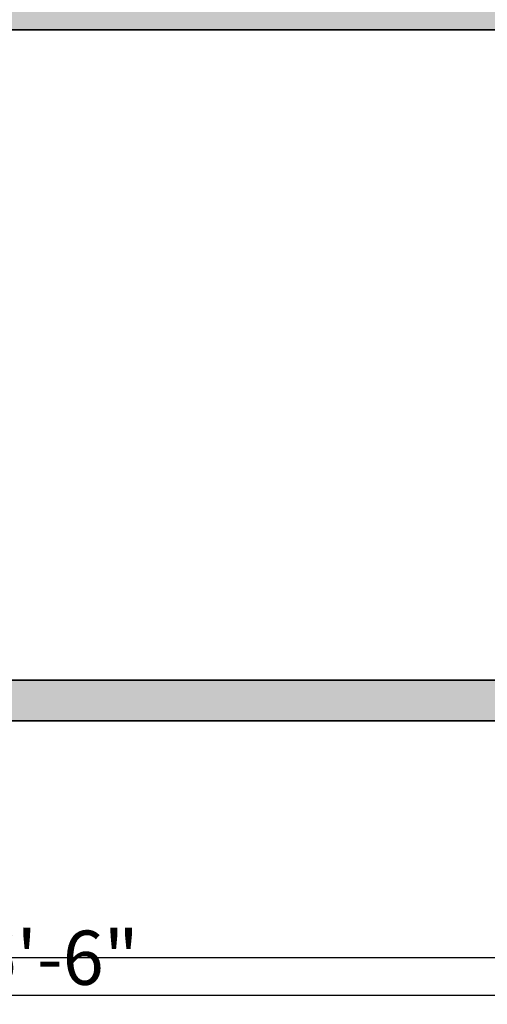
# Model space of a CAD drawing. Units: inches. Extents: x 2083 to 3317, y 1141 to 2115.
# Tile 84 of 256: x 2382 to 2486, y 1201 to 1419. Entities that reach past the tile are written whole.
import ezdxf

# ---------------------------------------------------------------- set-up
doc = ezdxf.new("R2010")
doc.units = ezdxf.units.IN
doc.layers.add('A-ANNO-DIMS', color=2, linetype='Continuous', lineweight=18)
doc.layers.add('A-WALL', color=7, linetype='Continuous', lineweight=35)
doc.layers.add('A-WALL-PATT', color=251, linetype='Continuous', lineweight=13, true_color=0x636466)
doc.styles.get("Standard").update_dxf_attribs({"font": 'arial.ttf'})
doc.dimstyles.new('ISO-25', dxfattribs={"dimtxt": 12, "dimasz": 12, "dimexe": 1.25, "dimexo": 0.625, "dimtad": 1, "dimlunit": 3, "dimtxsty": 'Standard', "dimcen": 2.5, "dimadec": 0, "dimazin": 0, "dimtfac": 1, "dimtmove": 0, "dimatfit": 3, "dimfxl": 1, "dimarcsym": 0})

# ---------------------------------------------------------------- blocks, each defined once
blk = doc.blocks.new('*D12')
at = {"layer": 'A-ANNO-DIMS', "color": 0, "lineweight": -2, "transparency": 16777216}
for p, q in [((2226.96, 1262.64), (2226.96, 1201.28)), ((2544.96, 1262.64), (2544.96, 1201.28)), ((2238.96, 1202.53), (2532.96, 1202.53))]:
    blk.add_line(p, q, dxfattribs=at)
at = {"layer": 'A-ANNO-DIMS', "color": 0, "transparency": 16777216}
for points in [[(2238.96, 1204.53), (2238.96, 1200.53), (2226.96, 1202.53)], [(2532.96, 1204.53), (2532.96, 1200.53), (2544.96, 1202.53)]]:
    blk.add_solid(points, dxfattribs=at)
at = {"layer": 'Defpoints', "color": 0, "transparency": 16777216}
for p in [(2226.96, 1263.26), (2544.96, 1263.26), (2544.96, 1202.53)]:
    blk.add_point(p, dxfattribs=at)
at = {"layer": 'A-ANNO-DIMS', "color": 0, "transparency": 16777216, "insert": (2385.96, 1209.29), "char_height": 12, "attachment_point": 5}
blk.add_mtext('26\'-6"', dxfattribs=at)
blk = doc.blocks.new('*D30')
at = {"layer": 'A-ANNO-DIMS', "color": 0, "lineweight": -2, "transparency": 16777216}
for p, q in [((2240.02, 1445.27), (2240.02, 1448.05)), ((2254.33, 1445.27), (2254.33, 1448.05)), ((2228.02, 1446.8), (2216.02, 1446.8)), ((2240.02, 1446.8), (2254.33, 1446.8)), ((2266.33, 1446.8), (2413.76, 1446.8))]:
    blk.add_line(p, q, dxfattribs=at)
at = {"layer": 'A-ANNO-DIMS', "color": 0, "transparency": 16777216}
for points in [[(2228.02, 1448.8), (2228.02, 1444.8), (2240.02, 1446.8)], [(2266.33, 1448.8), (2266.33, 1444.8), (2254.33, 1446.8)]]:
    blk.add_solid(points, dxfattribs=at)
at = {"layer": 'Defpoints', "color": 0, "transparency": 16777216}
for p in [(2254.33, 1446.8), (2240.02, 1444.65), (2254.33, 1444.65)]:
    blk.add_point(p, dxfattribs=at)
at = {"layer": 'A-ANNO-DIMS', "color": 0, "transparency": 16777216, "insert": (2346.05, 1453.63), "char_height": 12, "attachment_point": 5}
blk.add_mtext('WC 1\'-2 1/2" TYP.', dxfattribs=at)
blk = doc.blocks.new('*D34')
at = {"layer": 'A-ANNO-DIMS', "color": 0, "lineweight": -2, "transparency": 16777216}
for p, q in [((2226.96, 1262.64), (2226.96, 1209.66)), ((3126.96, 1262.64), (3126.96, 1209.66)), ((2238.96, 1210.91), (3114.96, 1210.91))]:
    blk.add_line(p, q, dxfattribs=at)
at = {"layer": 'A-ANNO-DIMS', "color": 0, "transparency": 16777216}
for points in [[(2238.96, 1212.91), (2238.96, 1208.91), (2226.96, 1210.91)], [(3114.96, 1212.91), (3114.96, 1208.91), (3126.96, 1210.91)]]:
    blk.add_solid(points, dxfattribs=at)
at = {"layer": 'Defpoints', "color": 0, "transparency": 16777216}
for p in [(2226.96, 1263.26), (3126.96, 1263.26), (3126.96, 1210.91)]:
    blk.add_point(p, dxfattribs=at)
at = {"layer": 'A-ANNO-DIMS', "color": 0, "transparency": 16777216, "insert": (2676.96, 1217.66), "char_height": 12, "attachment_point": 5}
blk.add_mtext('75\'-0"', dxfattribs=at)

msp = doc.modelspace()

# ---------------------------------------------------------------- hatches: boundary and pattern name
at = {"layer": 'A-WALL-PATT'}
h = msp.add_hatch(color=256, dxfattribs=at)
h.dxf.hatch_style = 1
h.paths.add_polyline_path([(3126.96, 2020.761), (2748.96, 2020.761), (2604.96, 2020.761), (2226.96, 2020.761), (2226.96, 1702.761), (2466.96, 1702.761), (2466.96, 1582.761), (2418.96, 1582.761), (2418.96, 1477.761), (2226.96, 1477.761), (2226.96, 1263.261), (2544.96, 1263.261), (2544.96, 1411.761), (2604.96, 1411.761), (2685.96, 1411.761), (2685.96, 1420.761), (2604.96, 1420.761), (2604.96, 1573.761), (2604.96, 1702.761), (2604.96, 2011.761), (2748.96, 2011.761), (2748.96, 1702.761), (2862.96, 1702.761), (2862.96, 1621.761), (2871.96, 1621.761), (2871.96, 1702.761), (2883.96, 1702.761), (2883.96, 1706.939, -0.0264593), (2883.96, 1711.761), (2757.96, 1711.761), (2757.96, 1807.761), (2787.96, 1807.761), (2787.96, 1812.261), (2757.96, 1812.261), (2757.96, 2011.761), (2877.96, 2011.761), (2877.96, 1812.261), (2847.96, 1812.261), (2847.96, 1807.761), (2889.836, 1807.761), (2889.836, 1812.261), (2882.46, 1812.261), (2882.46, 2011.761), (3117.96, 2011.761), (3117.96, 1812.261), (2937.836, 1812.261), (2937.836, 1807.761), (2995.71, 1807.761), (2995.71, 1796.118), (3000.21, 1796.118), (3000.21, 1807.761), (3117.96, 1807.761), (3117.96, 1711.761), (3000.21, 1711.761), (3000.21, 1760.118), (2998.573, 1760.118, -0.020711), (2995.71, 1760.118), (2995.71, 1711.761), (2931.96, 1711.761), (2931.96, 1702.761), (3126.96, 1702.761)])
h.paths.add_polyline_path([(2471.46, 2011.761), (2471.46, 1810.011), (2462.717, 1810.011), (2462.717, 1805.511), (2505.96, 1805.511), (2505.96, 1810.011), (2475.96, 1810.011), (2475.96, 2011.761), (2595.96, 2011.761), (2595.96, 1810.011), (2565.96, 1810.011), (2565.96, 1805.511), (2595.96, 1805.511), (2595.96, 1711.761), (2235.96, 1711.761), (2235.96, 1805.511), (2353.71, 1805.511), (2353.71, 1796.054), (2358.21, 1796.054), (2358.21, 1805.511), (2414.717, 1805.511), (2414.717, 1810.011), (2235.96, 1810.011), (2235.96, 2011.761)], flags=16)
h.paths.add_polyline_path([(2270.205, 1994.61), (2270.205, 1970.61), (2246.205, 1970.61), (2246.205, 1994.61)], flags=0)
edge = h.paths.add_edge_path(flags=0)
edge.add_ellipse((2332.027, 1899.798), major_axis=(-3.043, 3.043), ratio=0.1682525, start_angle=-161.33217, end_angle=-156.30711, ccw=False)
edge.add_ellipse((2333.082, 1898.744), major_axis=(-1.055, 1.055), ratio=0.4535321, start_angle=-123.37102, end_angle=-94.15911)
edge = h.paths.add_edge_path(flags=0)
edge.add_ellipse((2332.027, 1968.876), major_axis=(3.043, 3.043), ratio=0.1682525, start_angle=18.66783, end_angle=23.69289)
edge.add_spline(control_points=[(2332.926, 1970.691), (2332.227, 1970.336), (2330.894, 1969.659), (2328.413, 1970.932), (2327.204, 1967.749), (2324.71, 1969.956), (2322.533, 1967.012), (2320.013, 1971.296), (2317.68, 1968.158), (2316.041, 1967.102), (2315.427, 1966.81)], knot_values=[0, 0, 0, 0, 2.2670587, 4.3245589, 6.6855835, 8.8786411, 11.121502, 14.300359, 17.7552837, 19.732645, 19.732645, 19.732645, 19.732645], degree=3, periodic=0)
edge.add_ellipse((2332.027, 1968.876), major_axis=(3.043, 3.043), ratio=0.1682525, start_angle=18.66783, end_angle=23.69289, ccw=False)
edge.add_ellipse((2333.082, 1969.931), major_axis=(1.055, 1.055), ratio=0.4535321, start_angle=56.62898, end_angle=85.84089, ccw=False)
edge = h.paths.add_edge_path(flags=0)
edge.add_spline(control_points=[(2296.428, 1967.988), (2293.628, 1965.336), (2287.704, 1959.727), (2299.744, 1949.996), (2294.533, 1935.669), (2290.573, 1920.604), (2293.394, 1909.974), (2296.185, 1904.967)], knot_values=[0.0991853, 0.0991853, 0.0991853, 0.0991853, 0.3453009, 0.6198217, 0.9826526, 1.3860932, 1.8105546, 1.8105546, 1.8105546, 1.8105546], degree=3, periodic=0)
edge.add_spline(control_points=[(2296.185, 1904.967), (2297.384, 1902.619), (2298.001, 1901.949), (2298.553, 1901.468)], knot_values=[0.0062457, 0.0062457, 0.0062457, 0.0062457, 0.0554759, 0.0554759, 0.0554759, 0.0554759], degree=3, periodic=0)
edge.add_spline(control_points=[(2298.553, 1901.468), (2297.259, 1900.923), (2295.225, 1900.232), (2293.06, 1900.614), (2292.101, 1900.788), (2292.09, 1900.791)], knot_values=[0.3128349, 0.3128349, 0.3128349, 0.3128349, 0.4017797, 0.4749867, 0.4759027, 0.4759027, 0.4759027, 0.4759027], degree=3, periodic=0)
edge.add_arc((2292.794, 1904.664), 3.937, 215.4209, 259.69818, ccw=False)
edge.add_spline(control_points=[(2289.585, 1902.382), (2289.477, 1902.535), (2289.368, 1902.688), (2289.261, 1902.841)], knot_values=[0.1028719, 0.1028719, 0.1028719, 0.1028719, 0.1168958, 0.1168958, 0.1168958, 0.1168958], degree=3, periodic=0)
edge.add_spline(control_points=[(2289.261, 1902.841), (2288.687, 1902.55), (2287.64, 1902.02), (2285.881, 1901.874), (2283.853, 1901.504), (2281.72, 1899.711), (2278.467, 1899.493), (2276.157, 1901.883), (2272.259, 1899.804), (2267.778, 1901.843), (2262.244, 1900.184), (2257.415, 1901.782), (2254.318, 1900.726), (2253.178, 1900.337)], knot_values=[0, 0, 0, 0, 1.9079767, 3.4771759, 5.261074, 7.9728515, 11.6802485, 13.7179214, 16.9395917, 22.789562, 27.5025027, 33.5952153, 37.1456181, 37.1456181, 37.1456181, 37.1456181], degree=3, periodic=0)
edge.add_line((2253.178, 1900.337), (2250.244, 1902.841))
edge.add_line((2250.244, 1902.841), (2250.244, 1965.833))
edge.add_line((2250.244, 1965.833), (2253.178, 1968.337))
edge.add_spline(control_points=[(2253.178, 1968.337), (2254.318, 1967.948), (2257.415, 1966.892), (2262.244, 1968.49), (2267.778, 1966.831), (2271.527, 1968.537), (2273.876, 1967.828), (2274.207, 1967.728)], knot_values=[0, 0, 0, 0, 0.0901802, 0.2449351, 0.3646438, 0.5132331, 0.5378548, 0.5378548, 0.5378548, 0.5378548], degree=3, periodic=0)
edge.add_arc((2274.353, 1963.793), 3.937, 72.05113, 92.12795, ccw=False)
edge.add_arc((2281.297, 1985.23), 18.596, 252.05113, 288.56572)
edge.add_arc((2292.317, 1956.029), 12.646, 71.02679, 113.77822, ccw=False)
edge = h.paths.add_edge_path(flags=0)
edge.add_spline(control_points=[(2274.899, 1951.856), (2275.066, 1951.617), (2275.233, 1951.377), (2275.398, 1951.136)], knot_values=[1.4099157, 1.4099157, 1.4099157, 1.4099157, 1.4315903, 1.4315903, 1.4315903, 1.4315903], degree=3, periodic=0)
edge.add_spline(control_points=[(2275.398, 1951.136), (2275.792, 1950.562), (2276.179, 1949.984), (2276.546, 1949.397)], knot_values=[1.3582378, 1.3582378, 1.3582378, 1.3582378, 1.4099157, 1.4099157, 1.4099157, 1.4099157], degree=3, periodic=0)
edge.add_line((2276.546, 1949.397), (2277.437, 1947.862))
edge.add_spline(control_points=[(2277.437, 1947.862), (2276.304, 1945.673), (2274.64, 1942.427), (2274.632, 1938.094), (2272.799, 1930.852), (2274.356, 1943.897), (2275.948, 1947.923), (2276.546, 1949.397)], knot_values=[0.0056315, 0.0056315, 0.0056315, 0.0056315, 0.1860139, 0.2660015, 0.3570872, 0.5963902, 0.7397317, 0.7397317, 0.7397317, 0.7397317], degree=3, periodic=0)
edge.add_spline(control_points=[(2276.546, 1949.397), (2276.179, 1949.984), (2275.792, 1950.562), (2275.398, 1951.136)], knot_values=[1.3582378, 1.3582378, 1.3582378, 1.3582378, 1.4099157, 1.4099157, 1.4099157, 1.4099157], degree=3, periodic=0)
edge.add_spline(control_points=[(2275.398, 1951.136), (2274.943, 1950.08), (2274.208, 1948.025), (2273.935, 1944.851), (2272.469, 1937.627), (2273.466, 1945.696), (2274.701, 1951.059), (2274.899, 1951.856)], knot_values=[0.1043639, 0.1043639, 0.1043639, 0.1043639, 0.1896363, 0.2696239, 0.3607096, 0.6000126, 0.6446217, 0.6446217, 0.6446217, 0.6446217], degree=3, periodic=0)
h.paths.add_polyline_path([(2269.168, 1963.128, -0.3575267), (2268.171, 1960.976, -0.0925607), (2268.171, 1939.436, -0.3575267), (2269.168, 1937.285, -0.3575267), (2267.016, 1938.282, -0.1647847), (2254.686, 1938.282, -0.3575267), (2252.534, 1937.285, -0.3575267), (2253.531, 1939.436, -0.0925607), (2253.531, 1960.976, -0.3575267), (2252.534, 1963.128, -0.3575267), (2254.686, 1962.131, -0.1647847), (2267.016, 1962.131, -0.3575267)], flags=0)
h.paths.add_polyline_path([(2248.874, 1967.802), (2248.874, 1957.028), (2249.458, 1957.028), (2249.458, 1911.647), (2248.874, 1911.647), (2248.874, 1900.873), (2246.512, 1900.873, 0.1973271), (2244.15, 1902.457), (2244.15, 1966.218, 0.1973271), (2246.512, 1967.802)], flags=0)
h.paths.add_polyline_path([(2269.168, 1931.389, -0.3575267), (2268.171, 1929.238, -0.0925607), (2268.171, 1907.698, -0.3575267), (2269.168, 1905.547, -0.3575267), (2267.016, 1906.544, -0.1647847), (2254.686, 1906.544, -0.3575267), (2252.534, 1905.547, -0.3575267), (2253.531, 1907.698, -0.0925607), (2253.531, 1929.238, -0.3575267), (2252.534, 1931.389, -0.3575267), (2254.686, 1930.392, -0.1647847), (2267.016, 1930.392, -0.3575267)], flags=0)
edge = h.paths.add_edge_path(flags=0)
edge.add_spline(control_points=[(2276.197, 1906.724), (2276.168, 1909.029), (2276.114, 1913.372), (2270.598, 1924.925), (2273.905, 1919.013), (2275.922, 1916.262), (2275.475, 1912.402), (2277.258, 1910.381), (2276.696, 1908.225), (2276.646, 1906.813), (2276.618, 1906.008)], knot_values=[0, 0, 0, 0, 8.6102597, 16.2212739, 18.8430575, 23.8048978, 27.4408283, 29.3561016, 31.2034776, 33.6506866, 33.6506866, 33.6506866, 33.6506866], degree=3, periodic=0)
edge.add_spline(control_points=[(2276.618, 1906.008), (2276.623, 1905.624), (2276.498, 1904.629), (2275.442, 1903.855), (2274.937, 1903.08), (2274.859, 1902.841)], knot_values=[0.1564884, 0.1564884, 0.1564884, 0.1564884, 0.1843975, 0.2313765, 0.2505985, 0.2505985, 0.2505985, 0.2505985], degree=3, periodic=0)
edge.add_line((2274.859, 1902.841), (2276.506, 1902.841))
edge.add_spline(control_points=[(2276.506, 1902.841), (2276.788, 1903.085), (2277.665, 1904.125), (2278.25, 1904.341), (2277.654, 1908.527), (2278.156, 1906.228), (2278.1, 1905.286), (2278.847, 1904.069), (2277.857, 1903.415), (2277.874, 1902.991), (2277.904, 1902.841)], knot_values=[0.0595743, 0.0595743, 0.0595743, 0.0595743, 0.0807529, 0.1037415, 0.1697201, 0.1760361, 0.2071372, 0.2404744, 0.2623409, 0.2736605, 0.2736605, 0.2736605, 0.2736605], degree=3, periodic=0)
edge.add_line((2277.904, 1902.841), (2280.03, 1902.841))
edge.add_spline(control_points=[(2280.03, 1902.841), (2279.888, 1903.088), (2279.499, 1903.982), (2280.152, 1905.939), (2278.104, 1909.658), (2279.762, 1907.185), (2280.328, 1904.875), (2280.485, 1903.49), (2281.463, 1903.249), (2281.758, 1902.936), (2281.834, 1902.841)], knot_values=[0.013856, 0.013856, 0.013856, 0.013856, 0.0348738, 0.0888667, 0.1078792, 0.1267378, 0.158714, 0.1937575, 0.2174868, 0.2267221, 0.2267221, 0.2267221, 0.2267221], degree=3, periodic=0)
edge.add_spline(control_points=[(2281.834, 1902.841), (2281.788, 1902.827), (2281.647, 1902.783), (2281.396, 1902.859), (2281.088, 1902.985), (2280.721, 1903.061), (2280.333, 1903.026), (2280.125, 1902.899), (2280.03, 1902.841)], knot_values=[0, 0, 0, 0, 0.1441304, 0.435517, 0.7492759, 1.1530457, 1.5483707, 1.878348, 1.878348, 1.878348, 1.878348], degree=3, periodic=0)
edge.add_line((2280.03, 1902.841), (2277.904, 1902.841))
edge.add_spline(control_points=[(2277.904, 1902.841), (2277.893, 1902.796), (2277.865, 1902.68), (2277.607, 1902.687), (2277.274, 1902.801), (2276.838, 1902.62), (2276.584, 1902.789), (2276.506, 1902.841)], knot_values=[0, 0, 0, 0, 0.1271885, 0.3261988, 0.6280094, 1.2435704, 1.5153306, 1.5153306, 1.5153306, 1.5153306], degree=3, periodic=0)
edge.add_line((2276.506, 1902.841), (2274.859, 1902.841))
edge.add_spline(control_points=[(2274.859, 1902.841), (2274.814, 1902.899), (2274.725, 1903.013), (2274.493, 1903.119), (2274.244, 1902.961), (2273.937, 1903.185), (2273.614, 1902.983), (2273.408, 1902.883), (2273.322, 1902.841)], knot_values=[0, 0, 0, 0, 0.2184302, 0.4369566, 0.6879766, 0.9903786, 1.3983955, 1.6918498, 1.6918498, 1.6918498, 1.6918498], degree=3, periodic=0)
edge.add_spline(control_points=[(2273.322, 1902.841), (2273.617, 1903.446), (2274.274, 1904.538), (2276.027, 1904.574), (2276.207, 1906.584), (2276.197, 1906.724)], knot_values=[0.0122268, 0.0122268, 0.0122268, 0.0122268, 0.0594721, 0.1062177, 0.134458, 0.134458, 0.134458, 0.134458], degree=3, periodic=0)
h.paths.add_polyline_path([(2270.776, 1897.79), (2270.776, 1873.79), (2246.776, 1873.79), (2246.776, 1897.79)], flags=0)
h.paths.add_polyline_path([(2353.71, 1760.005), (2353.71, 1760.054), (2358.21, 1760.054, -0.033729)], flags=0)
h.paths.add_polyline_path([(2321.819, 1737.529), (2341.995, 1737.529, -0.4142136), (2343.203, 1736.321), (2343.203, 1721.021, -0.4142136), (2341.995, 1719.813), (2321.819, 1719.813, -0.4142136), (2320.611, 1721.021), (2320.611, 1736.321, -0.4142136)], flags=0)
h.paths.add_polyline_path([(2324.235, 1736.321), (2339.579, 1736.321, -0.4142136), (2341.995, 1733.905), (2341.995, 1725.45, -0.4142136), (2339.579, 1723.034), (2333.681, 1723.034), (2333.845, 1722.045, -0.8706461), (2335.425, 1721.826, -0.767327), (2333.923, 1721.423), (2331.291, 1721.423, -0.767327), (2329.788, 1721.826, -0.8706461), (2331.368, 1722.045), (2331.533, 1723.034), (2324.235, 1723.034, -0.4142136), (2321.819, 1725.45), (2321.819, 1733.905, -0.4142136)], flags=0)
h.paths.add_polyline_path([(2570.484, 1928.615), (2589.684, 1928.615), (2590.169, 1928.615), (2590.169, 1904.993), (2570.484, 1904.993)], flags=0)
h.paths.add_polyline_path([(2574.447, 1927.264, -1), (2572.829, 1927.264, -1)], flags=0)
h.paths.add_polyline_path([(2573.09, 1926.941), (2573.925, 1927.776), (2574.148, 1927.553), (2573.313, 1926.718)], flags=0)
h.paths.add_polyline_path([(2578.779, 1919.73, -1), (2571.592, 1919.73, -1)], flags=0)
h.paths.add_polyline_path([(2578.385, 1919.73, -1), (2571.985, 1919.73, -1)], flags=0)
h.paths.add_polyline_path([(2331.596, 1729.476, -1), (2333.618, 1729.476, -1)], flags=0)
h.paths.add_polyline_path([(2578.034, 1927.264, -1), (2576.416, 1927.264, -1)], flags=0)
h.paths.add_polyline_path([(2576.689, 1927.531), (2576.912, 1927.754), (2577.747, 1926.919), (2577.524, 1926.696)], flags=0)
h.paths.add_polyline_path([(2578.139, 1909.86, -1), (2572.232, 1909.86, -1)], flags=0)
h.paths.add_polyline_path([(2577.745, 1909.86, -1), (2572.625, 1909.86, -1)], flags=0)
h.paths.add_polyline_path([(2583.798, 1927.264, -1), (2582.179, 1927.264, -1)], flags=0)
h.paths.add_polyline_path([(2582.719, 1927.754), (2583.554, 1926.919), (2583.331, 1926.696), (2582.496, 1927.531)], flags=0)
h.paths.add_polyline_path([(2582.496, 1927.531), (2582.719, 1927.754), (2583.554, 1926.919), (2583.331, 1926.696)], flags=0)
h.paths.add_polyline_path([(2587.739, 1920.53, -1), (2581.832, 1920.53, -1)], flags=0)
h.paths.add_polyline_path([(2587.345, 1920.53, -1), (2582.225, 1920.53, -1)], flags=0)
h.paths.add_polyline_path([(2587.385, 1927.264, -1), (2585.766, 1927.264, -1)], flags=0)
h.paths.add_polyline_path([(2586.082, 1926.98), (2586.917, 1927.815), (2587.14, 1927.593), (2586.305, 1926.758)], flags=0)
h.paths.add_polyline_path([(2588.379, 1910.66, -1), (2581.192, 1910.66, -1)], flags=0)
h.paths.add_polyline_path([(2587.985, 1910.66, -1), (2581.585, 1910.66, -1)], flags=0)
h.paths.add_polyline_path([(2417.168, 1729.478), (2437.344, 1729.478, -0.4142136), (2438.552, 1728.27), (2438.552, 1712.969, -0.4142136), (2437.344, 1711.761), (2417.168, 1711.761, -0.4142136), (2415.96, 1712.969), (2415.96, 1728.27, -0.4142136)], flags=0)
h.paths.add_polyline_path([(2419.584, 1728.27), (2434.928, 1728.27, -0.4142136), (2437.344, 1725.854), (2437.344, 1717.398, -0.4142136), (2434.928, 1714.983), (2429.029, 1714.983), (2429.194, 1713.994, -0.8706461), (2430.774, 1713.775, -0.767327), (2429.271, 1713.372), (2426.64, 1713.372, -0.767327), (2425.137, 1713.775, -0.8706461), (2426.717, 1713.994), (2426.882, 1714.983), (2419.584, 1714.983, -0.4142136), (2417.168, 1717.398), (2417.168, 1725.854, -0.4142136)], flags=0)
h.paths.add_polyline_path([(2419.584, 1728.27), (2434.928, 1728.27, -0.4142136), (2437.344, 1725.854), (2437.344, 1717.398, -0.4142136), (2434.928, 1714.983), (2429.029, 1714.983), (2428.358, 1719.009), (2427.553, 1719.009), (2426.882, 1714.983), (2419.584, 1714.983, -0.4142136), (2417.168, 1717.398), (2417.168, 1725.854, -0.4142136)], flags=0)
h.paths.add_polyline_path([(2426.944, 1721.425, -1), (2428.967, 1721.425, -1)], flags=0)
h.paths.add_polyline_path([(2475.96, 1702.761), (2595.96, 1702.761), (2595.96, 1582.761), (2475.96, 1582.761)], flags=16)
h.paths.add_polyline_path([(2427.96, 1573.761), (2595.96, 1573.761), (2595.96, 1468.761), (2595.96, 1420.761), (2384.46, 1420.761), (2384.46, 1468.761), (2427.96, 1468.761)], flags=16)
h.paths.add_polyline_path([(2379.96, 1468.761), (2379.96, 1420.761), (2235.96, 1420.761), (2235.96, 1468.761)], flags=16)
h.paths.add_polyline_path([(2317.816, 1466.696), (2337.992, 1466.696, -0.4142136), (2339.2, 1465.488), (2339.2, 1450.187, -0.4142136), (2337.992, 1448.979), (2317.816, 1448.979, -0.4142136), (2316.608, 1450.187), (2316.608, 1465.488, -0.4142136)], flags=0)
h.paths.add_polyline_path([(2320.232, 1465.488), (2335.576, 1465.488, -0.4142136), (2337.992, 1463.072), (2337.992, 1454.616, -0.4142136), (2335.576, 1452.2), (2329.677, 1452.2), (2329.842, 1451.212, -0.8706461), (2331.422, 1450.992, -0.767327), (2329.92, 1450.59), (2327.288, 1450.59, -0.767327), (2325.785, 1450.992, -0.8706461), (2327.365, 1451.212), (2327.53, 1452.2), (2320.232, 1452.2, -0.4142136), (2317.816, 1454.616), (2317.816, 1463.072, -0.4142136)], flags=0)
h.paths.add_polyline_path([(2320.232, 1465.488), (2335.576, 1465.488, -0.4142136), (2337.992, 1463.072), (2337.992, 1454.616, -0.4142136), (2335.576, 1452.2), (2329.677, 1452.2), (2329.006, 1456.227), (2328.201, 1456.227), (2327.53, 1452.2), (2320.232, 1452.2, -0.4142136), (2317.816, 1454.616), (2317.816, 1463.072, -0.4142136)], flags=0)
h.paths.add_polyline_path([(2327.593, 1458.643, -1), (2329.615, 1458.643, -1)], flags=0)
h.paths.add_polyline_path([(2244.412, 1433.34), (2241.921, 1433.34, -0.4142136), (2240.018, 1435.244), (2240.018, 1440.953, -0.4142105), (2241.921, 1442.856), (2244.412, 1442.856, -1.9764724)], flags=0)
h.paths.add_polyline_path([(2245.357, 1434.398, -0.4142136), (2245.357, 1441.799, -2.1440985)], flags=0)
h.paths.add_polyline_path([(2535.96, 1416.261), (2535.96, 1272.261), (2235.96, 1272.261), (2235.96, 1416.261)], flags=16)
h.paths.add_polyline_path([(2260.12, 1384.293), (2260.12, 1362.039), (2237.865, 1362.039), (2237.865, 1384.293)], flags=0)
edge = h.paths.add_edge_path(flags=0)
edge.add_line((2318.252, 1362.093), (2318.146, 1362.001))
edge.add_ellipse((2317.445, 1360.431), major_axis=(2.822, 2.822), ratio=0.1682525, start_angle=18.66783, end_angle=20.94813, ccw=False)
edge.add_ellipse((2318.423, 1361.409), major_axis=(0.978, 0.978), ratio=0.4535321, start_angle=56.62898, end_angle=70.2262, ccw=False)
edge = h.paths.add_edge_path(flags=0)
edge.add_line((2319.107, 1295.571), (2319.015, 1295.677))
edge.add_ellipse((2317.445, 1296.378), major_axis=(-2.822, 2.822), ratio=0.1682525, start_angle=-161.33217, end_angle=-159.05187, ccw=False)
edge.add_ellipse((2318.423, 1295.4), major_axis=(-0.978, 0.978), ratio=0.4535321, start_angle=-123.37102, end_angle=-109.7738)
edge = h.paths.add_edge_path(flags=0)
edge.add_spline(control_points=[(2284.21, 1301.17), (2284.581, 1300.445), (2284.891, 1299.892), (2285.16, 1299.461)], knot_values=[0.0390658, 0.0390658, 0.0390658, 0.0390658, 0.0554759, 0.0554759, 0.0554759, 0.0554759], degree=3, periodic=0)
edge.add_line((2285.16, 1299.461), (2284.21, 1301.17))
edge = h.paths.add_edge_path(flags=0)
edge.add_line((2280.412, 1297.298), (2283.37, 1297.036))
edge.add_line((2283.37, 1297.036), (2286.406, 1297.926))
edge.add_spline(control_points=[(2286.406, 1297.926), (2285.305, 1297.463), (2284.345, 1297.129), (2283.37, 1297.036)], knot_values=[0.3943688, 0.3943688, 0.3943688, 0.3943688, 0.4759027, 0.4759027, 0.4759027, 0.4759027], degree=3, periodic=0)
edge.add_spline(control_points=[(2283.37, 1297.036), (2283.281, 1297.028), (2282.316, 1296.957), (2281.313, 1297.134), (2280.423, 1297.296), (2280.412, 1297.298)], knot_values=[0.3128349, 0.3128349, 0.3128349, 0.3128349, 0.3202458, 0.3934528, 0.3943688, 0.3943688, 0.3943688, 0.3943688], degree=3, periodic=0)
edge = h.paths.add_edge_path(flags=0)
edge.add_line((2284.436, 1359.607), (2280.446, 1355.328))
edge.add_line((2280.446, 1355.328), (2279.58, 1351.018))
edge.add_line((2279.58, 1351.018), (2282.413, 1346.58))
edge.add_spline(control_points=[(2282.413, 1346.58), (2283.153, 1345.589), (2284.253, 1344.029), (2284.801, 1342.387), (2284.935, 1341.806)], knot_values=[1.2400982, 1.2400982, 1.2400982, 1.2400982, 1.3328922, 1.3827123, 1.3827123, 1.3827123, 1.3827123], degree=3, periodic=0)
edge.add_spline(control_points=[(2284.935, 1341.806), (2285.319, 1340.141), (2285.233, 1338.409), (2284.91, 1336.654)], knot_values=[1.0974841, 1.0974841, 1.0974841, 1.0974841, 1.2400982, 1.2400982, 1.2400982, 1.2400982], degree=3, periodic=0)
edge.add_spline(control_points=[(2284.91, 1336.654), (2284.587, 1334.899), (2284.027, 1333.12), (2283.463, 1331.361)], knot_values=[0.9548699, 0.9548699, 0.9548699, 0.9548699, 1.0974841, 1.0974841, 1.0974841, 1.0974841], degree=3, periodic=0)
edge.add_line((2283.463, 1331.361), (2281.89, 1326.153))
edge.add_line((2281.89, 1326.153), (2280.756, 1321.056))
edge.add_line((2280.756, 1321.056), (2280.299, 1316.002))
edge.add_line((2280.299, 1316.002), (2280.716, 1310.95))
edge.add_line((2280.716, 1310.95), (2282.028, 1305.972))
edge.add_line((2282.028, 1305.972), (2284.21, 1301.17))
edge.add_spline(control_points=[(2284.21, 1301.17), (2283.341, 1302.73), (2282.612, 1304.336), (2282.028, 1305.972)], knot_values=[0.0991853, 0.0991853, 0.0991853, 0.0991853, 0.2417994, 0.2417994, 0.2417994, 0.2417994], degree=3, periodic=0)
edge.add_spline(control_points=[(2282.028, 1305.972), (2281.444, 1307.608), (2281.005, 1309.273), (2280.716, 1310.95)], knot_values=[0.2417994, 0.2417994, 0.2417994, 0.2417994, 0.3844135, 0.3844135, 0.3844135, 0.3844135], degree=3, periodic=0)
edge.add_spline(control_points=[(2280.716, 1310.95), (2280.433, 1312.588), (2280.289, 1314.277), (2280.299, 1315.962), (2280.299, 1316.002)], knot_values=[0.3844135, 0.3844135, 0.3844135, 0.3844135, 0.5236467, 0.5270276, 0.5270276, 0.5270276, 0.5270276], degree=3, periodic=0)
edge.add_spline(control_points=[(2280.299, 1316.002), (2280.312, 1317.687), (2280.478, 1319.368), (2280.756, 1321.056)], knot_values=[0.5270276, 0.5270276, 0.5270276, 0.5270276, 0.6696417, 0.6696417, 0.6696417, 0.6696417], degree=3, periodic=0)
edge.add_spline(control_points=[(2280.756, 1321.056), (2281.035, 1322.744), (2281.426, 1324.44), (2281.89, 1326.153)], knot_values=[0.6696417, 0.6696417, 0.6696417, 0.6696417, 0.8122558, 0.8122558, 0.8122558, 0.8122558], degree=3, periodic=0)
edge.add_spline(control_points=[(2281.89, 1326.153), (2282.264, 1327.533), (2282.788, 1329.262), (2283.353, 1331.018), (2283.463, 1331.361)], knot_values=[0.8122558, 0.8122558, 0.8122558, 0.8122558, 0.9270873, 0.9548699, 0.9548699, 0.9548699, 0.9548699], degree=3, periodic=0)
edge.add_line((2283.463, 1331.361), (2284.91, 1336.654))
edge.add_line((2284.91, 1336.654), (2284.935, 1341.806))
edge.add_line((2284.935, 1341.806), (2282.413, 1346.58))
edge.add_spline(control_points=[(2282.413, 1346.58), (2281.275, 1348.104), (2280.078, 1349.57), (2279.58, 1351.018)], knot_values=[1.3827123, 1.3827123, 1.3827123, 1.3827123, 1.5253264, 1.5253264, 1.5253264, 1.5253264], degree=3, periodic=0)
edge.add_spline(control_points=[(2279.58, 1351.018), (2279.443, 1351.415), (2279.136, 1352.857), (2279.735, 1354.29), (2280.446, 1355.328)], knot_values=[1.5253264, 1.5253264, 1.5253264, 1.5253264, 1.564439, 1.6679405, 1.6679405, 1.6679405, 1.6679405], degree=3, periodic=0)
edge.add_spline(control_points=[(2280.446, 1355.328), (2281.426, 1356.758), (2282.931, 1358.183), (2284.436, 1359.607)], knot_values=[1.6679405, 1.6679405, 1.6679405, 1.6679405, 1.8105546, 1.8105546, 1.8105546, 1.8105546], degree=3, periodic=0)
edge.add_arc((2280.623, 1348.518), 11.726, 71.02679, 113.77822)
edge.add_arc((2270.405, 1375.595), 17.244, 252.05113, 288.56572, ccw=False)
edge.add_arc((2263.966, 1355.718), 3.651, 72.05113, 92.12795)
edge.add_arc((2263.966, 1355.718), 3.651, 92.12795, 177.98513)
edge.add_spline(control_points=[(2260.318, 1355.846), (2260.26, 1354.221), (2260.551, 1350.187), (2262.999, 1346.766), (2264.473, 1344.649)], knot_values=[1.4315903, 1.4315903, 1.4315903, 1.4315903, 1.5641438, 1.7706953, 1.7706953, 1.7706953, 1.7706953], degree=3, periodic=0)
edge.add_line((2264.473, 1344.649), (2264.936, 1343.983))
edge.add_spline(control_points=[(2263.801, 1340.248), (2263.843, 1340.514), (2264.067, 1341.756), (2264.513, 1343.002), (2264.935, 1343.981)], knot_values=[0.5365702, 0.5365702, 0.5365702, 0.5365702, 0.5593494, 0.6446217, 0.6446217, 0.6446217, 0.6446217], degree=3, periodic=0)
edge.add_spline(control_points=[(2264.935, 1343.981), (2265.118, 1343.715), (2265.299, 1343.448), (2265.477, 1343.179)], knot_values=[1.3840767, 1.3840767, 1.3840767, 1.3840767, 1.4099157, 1.4099157, 1.4099157, 1.4099157], degree=3, periodic=0)
edge.add_spline(control_points=[(2265.477, 1343.179), (2265.655, 1342.911), (2265.829, 1342.641), (2265.999, 1342.369)], knot_values=[1.3582378, 1.3582378, 1.3582378, 1.3582378, 1.3840767, 1.3840767, 1.3840767, 1.3840767], degree=3, periodic=0)
edge.add_line((2265.999, 1342.369), (2266.826, 1340.946))
edge.add_spline(control_points=[(2266.826, 1340.946), (2268.894, 1337.09), (2271.398, 1325.843), (2270.516, 1310.569), (2275.919, 1301.861), (2277.79, 1299.199)], knot_values=[0.1168958, 0.1168958, 0.1168958, 0.1168958, 0.4729873, 1.0509689, 1.3137934, 1.3137934, 1.3137934, 1.3137934], degree=3, periodic=0)
edge.add_spline(control_points=[(2277.79, 1299.199), (2277.839, 1299.128), (2277.889, 1299.057), (2277.94, 1298.987)], knot_values=[0.1098839, 0.1098839, 0.1098839, 0.1098839, 0.1168958, 0.1168958, 0.1168958, 0.1168958], degree=3, periodic=0)
edge.add_line((2277.94, 1298.987), (2277.789, 1299.199))
edge.add_spline(control_points=[(2277.789, 1299.199), (2277.257, 1298.929), (2276.286, 1298.438), (2275.039, 1298.334), (2274.383, 1298.239), (2274.215, 1298.209)], knot_values=[33.1218702, 33.1218702, 33.1218702, 33.1218702, 35.0290557, 36.5982549, 37.1448269, 37.1448269, 37.1448269, 37.1448269], degree=3, periodic=0)
edge.add_line((2274.215, 1298.209), (2273.073, 1297.893))
edge.add_spline(control_points=[(2273.073, 1297.893), (2272.323, 1297.58), (2271.039, 1296.511), (2269.248, 1296.226), (2268.423, 1296.375)], knot_values=[26.5325843, 26.5325843, 26.5325843, 26.5325843, 29.198919, 31.8391012, 31.8391012, 31.8391012, 31.8391012], degree=3, periodic=0)
edge.add_line((2268.423, 1296.375), (2263.879, 1297.458))
edge.add_spline(control_points=[(2263.879, 1297.458), (2263.556, 1297.359), (2261.86, 1296.839), (2260.239, 1297.282), (2258.933, 1297.516)], knot_values=[15.9195506, 15.9195506, 15.9195506, 15.9195506, 16.9395917, 21.2260675, 21.2260675, 21.2260675, 21.2260675], degree=3, periodic=0)
edge.add_line((2258.933, 1297.516), (2254.055, 1297.329))
edge.add_spline(control_points=[(2254.055, 1297.329), (2253.756, 1297.296), (2252.114, 1297.165), (2250.462, 1297.544), (2249.13, 1297.668)], knot_values=[5.3065169, 5.3065169, 5.3065169, 5.3065169, 6.2764352, 10.6130337, 10.6130337, 10.6130337, 10.6130337], degree=3, periodic=0)
edge.add_line((2249.13, 1297.668), (2244.332, 1296.878))
edge.add_line((2244.332, 1296.878), (2241.611, 1299.199))
edge.add_line((2241.611, 1299.199), (2241.611, 1357.609))
edge.add_line((2241.611, 1357.609), (2244.332, 1359.931))
edge.add_line((2244.332, 1359.931), (2252.729, 1359.543))
edge.add_spline(control_points=[(2252.729, 1359.543), (2252.871, 1359.546), (2253.306, 1359.548), (2253.74, 1359.514), (2254.032, 1359.482)], knot_values=[0.233291, 0.233291, 0.233291, 0.233291, 0.2449351, 0.2689274, 0.2689274, 0.2689274, 0.2689274], degree=3, periodic=0)
edge.add_line((2254.032, 1359.482), (2259.587, 1359.416))
edge.add_spline(control_points=[(2259.587, 1359.416), (2260.677, 1359.629), (2262.073, 1359.897), (2263.524, 1359.459), (2263.83, 1359.366)], knot_values=[0.4225164, 0.4225164, 0.4225164, 0.4225164, 0.5132331, 0.5378548, 0.5378548, 0.5378548, 0.5378548], degree=3, periodic=0)
edge.add_arc((2263.966, 1355.718), 3.651, 72.05113, 92.12795, ccw=False)
edge.add_arc((2270.405, 1375.595), 17.244, 252.05113, 288.56572)
edge.add_arc((2280.623, 1348.518), 11.726, 71.02679, 113.77822, ccw=False)
h.paths.add_polyline_path([(2240.341, 1359.435), (2240.341, 1349.444), (2240.882, 1349.444), (2240.882, 1307.365), (2240.341, 1307.365), (2240.341, 1297.374), (2238.15, 1297.374, 0.1973271), (2235.96, 1298.843), (2235.96, 1357.966, 0.1973271), (2238.15, 1359.435)], flags=0)
h.paths.add_polyline_path([(2259.158, 1355.101, -0.3575267), (2258.233, 1353.106, -0.0925607), (2258.233, 1333.133, -0.3575267), (2259.158, 1331.138, -0.3575267), (2257.163, 1332.062, -0.1647847), (2245.729, 1332.062, -0.3575267), (2243.735, 1331.138, -0.3575267), (2244.659, 1333.133, -0.0925607), (2244.659, 1353.106, -0.3575267), (2243.735, 1355.101, -0.3575267), (2245.729, 1354.176, -0.1647847), (2257.163, 1354.176, -0.3575267)], flags=0)
edge = h.paths.add_edge_path(flags=0)
edge.add_line((2265.999, 1342.369), (2266.826, 1340.946))
edge.add_line((2266.826, 1340.946), (2265.308, 1337.814))
edge.add_line((2265.308, 1337.814), (2264.358, 1334.653))
edge.add_line((2264.358, 1334.653), (2264.262, 1333.8))
edge.add_spline(control_points=[(2264.262, 1333.8), (2264.208, 1333.187), (2264.162, 1332.366), (2264.007, 1331.414), (2263.969, 1331.202)], knot_values=[0.4644442, 0.4644442, 0.4644442, 0.4644442, 0.5166905, 0.5316081, 0.5316081, 0.5316081, 0.5316081], degree=3, periodic=0)
edge.add_spline(control_points=[(2263.969, 1331.202), (2263.775, 1330.119), (2263.424, 1328.791), (2263.257, 1328.531), (2263.234, 1328.515)], knot_values=[0.3726816, 0.3726816, 0.3726816, 0.3726816, 0.4488497, 0.4644442, 0.4644442, 0.4644442, 0.4644442], degree=3, periodic=0)
edge.add_spline(control_points=[(2263.234, 1328.515), (2263.096, 1328.42), (2263.131, 1329.301), (2263.275, 1330.616)], knot_values=[0.2809191, 0.2809191, 0.2809191, 0.2809191, 0.3726816, 0.3726816, 0.3726816, 0.3726816], degree=3, periodic=0)
edge.add_spline(control_points=[(2263.275, 1330.616), (2263.419, 1331.93), (2263.672, 1333.677), (2263.97, 1335.315)], knot_values=[0.1891566, 0.1891566, 0.1891566, 0.1891566, 0.2809191, 0.2809191, 0.2809191, 0.2809191], degree=3, periodic=0)
edge.add_spline(control_points=[(2263.97, 1335.315), (2264.1, 1336.032), (2264.419, 1337.622), (2264.755, 1338.864), (2264.947, 1339.491)], knot_values=[0.097394, 0.097394, 0.097394, 0.097394, 0.1375775, 0.1891566, 0.1891566, 0.1891566, 0.1891566], degree=3, periodic=0)
edge.add_spline(control_points=[(2264.947, 1339.491), (2265.29, 1340.606), (2265.644, 1341.494), (2265.999, 1342.369)], knot_values=[0.0056315, 0.0056315, 0.0056315, 0.0056315, 0.097394, 0.097394, 0.097394, 0.097394], degree=3, periodic=0)
h.paths.add_polyline_path([(2259.158, 1325.671, -0.3575267), (2258.233, 1323.676, -0.0925607), (2258.233, 1303.703, -0.3575267), (2259.158, 1301.708, -0.3575267), (2257.163, 1302.633, -0.1647847), (2245.729, 1302.633, -0.3575267), (2243.735, 1301.708, -0.3575267), (2244.659, 1303.703, -0.0925607), (2244.659, 1323.676, -0.3575267), (2243.735, 1325.671, -0.3575267), (2245.729, 1324.747, -0.1647847), (2257.163, 1324.747, -0.3575267)], flags=0)
edge = h.paths.add_edge_path(flags=0)
edge.add_spline(control_points=[(2261.709, 1317.311), (2261.679, 1317.418), (2261.762, 1317.389), (2262.491, 1316.09), (2262.962, 1315.301)], knot_values=[14.9558607, 14.9558607, 14.9558607, 14.9558607, 16.2212739, 18.6948259, 18.6948259, 18.6948259, 18.6948259], degree=3, periodic=0)
edge.add_spline(control_points=[(2262.962, 1315.301), (2262.99, 1315.254), (2263.702, 1314.067), (2264.349, 1313.127), (2264.73, 1312.164)], knot_values=[18.6948259, 18.6948259, 18.6948259, 18.6948259, 18.8430575, 22.433791, 22.433791, 22.433791, 22.433791], degree=3, periodic=0)
edge.add_spline(control_points=[(2264.73, 1312.164), (2264.876, 1311.796), (2265.177, 1310.77), (2265.143, 1309.559), (2265.248, 1308.824)], knot_values=[22.433791, 22.433791, 22.433791, 22.433791, 23.8048978, 26.1727562, 26.1727562, 26.1727562, 26.1727562], degree=3, periodic=0)
edge.add_line((2265.248, 1308.824), (2265.851, 1307.172))
edge.add_spline(control_points=[(2265.851, 1307.172), (2266.065, 1306.822), (2266.384, 1306.332), (2266.424, 1305.781), (2266.42, 1305.611)], knot_values=[28.0625624, 28.0625624, 28.0625624, 28.0625624, 29.3561016, 29.9117214, 29.9117214, 29.9117214, 29.9117214], degree=3, periodic=0)
edge.add_spline(control_points=[(2266.42, 1305.611), (2266.416, 1305.433), (2266.394, 1305.25), (2266.365, 1305.066)], knot_values=[29.9117214, 29.9117214, 29.9117214, 29.9117214, 30.4978371, 30.4978371, 30.4978371, 30.4978371], degree=3, periodic=0)
edge.add_line((2266.365, 1305.066), (2266.066, 1302.136))
edge.add_spline(control_points=[(2266.066, 1302.136), (2266.071, 1301.78), (2265.998, 1301.2), (2265.663, 1300.759), (2265.509, 1300.586)], knot_values=[0.1564884, 0.1564884, 0.1564884, 0.1564884, 0.1843975, 0.2035434, 0.2035434, 0.2035434, 0.2035434], degree=3, periodic=0)
edge.add_line((2265.509, 1300.586), (2264.435, 1299.199))
edge.add_line((2264.435, 1299.199), (2265.962, 1299.199))
edge.add_line((2265.962, 1299.199), (2267.336, 1301.175))
edge.add_line((2267.336, 1301.175), (2267.312, 1301.986))
edge.add_spline(control_points=[(2267.312, 1301.986), (2267.261, 1302.862), (2267.16, 1303.737), (2267.271, 1303.326)], knot_values=[0.1262286, 0.1262286, 0.1262286, 0.1262286, 0.1666174, 0.1666174, 0.1666174, 0.1666174], degree=3, periodic=0)
edge.add_spline(control_points=[(2267.271, 1303.326), (2267.28, 1303.294), (2267.31, 1303.175), (2267.373, 1302.884), (2267.406, 1302.683), (2267.418, 1302.601)], knot_values=[0.1666174, 0.1666174, 0.1666174, 0.1666174, 0.1697201, 0.1760361, 0.1807647, 0.1807647, 0.1807647, 0.1807647], degree=3, periodic=0)
edge.add_spline(control_points=[(2267.744, 1300.988), (2267.688, 1301.151), (2267.481, 1301.657), (2267.484, 1302.145), (2267.418, 1302.601)], knot_values=[0.1807647, 0.1807647, 0.1807647, 0.1807647, 0.1937665, 0.2201389, 0.2201389, 0.2201389, 0.2201389], degree=3, periodic=0)
edge.add_line((2267.418, 1302.601), (2267.744, 1300.988))
edge.add_spline(control_points=[(2267.744, 1300.988), (2267.832, 1300.732), (2267.932, 1300.31), (2267.555, 1299.975), (2267.429, 1299.829)], knot_values=[0.2201389, 0.2201389, 0.2201389, 0.2201389, 0.2404744, 0.2548903, 0.2548903, 0.2548903, 0.2548903], degree=3, periodic=0)
edge.add_line((2267.429, 1299.829), (2267.258, 1299.199))
edge.add_line((2267.258, 1299.199), (2269.23, 1299.199))
edge.add_spline(control_points=[(2269.23, 1299.199), (2269.099, 1299.429), (2268.843, 1300.016), (2269.012, 1300.916), (2268.947, 1301.661)], knot_values=[0.013856, 0.013856, 0.013856, 0.013856, 0.0348738, 0.0670726, 0.0670726, 0.0670726, 0.0670726], degree=3, periodic=0)
edge.add_line((2268.947, 1301.661), (2268.432, 1303.603))
edge.add_spline(control_points=[(2268.432, 1303.603), (2268.176, 1304.192), (2267.596, 1305.251), (2268.041, 1304.623), (2268.251, 1304.282)], knot_values=[0.0901547, 0.0901547, 0.0901547, 0.0901547, 0.1078792, 0.1202891, 0.1202891, 0.1202891, 0.1202891], degree=3, periodic=0)
edge.add_spline(control_points=[(2268.251, 1304.282), (2268.361, 1304.105), (2269.058, 1302.918), (2269.383, 1301.59), (2269.521, 1300.776), (2269.575, 1300.556)], knot_values=[0.1202891, 0.1202891, 0.1202891, 0.1202891, 0.1267378, 0.158714, 0.1735056, 0.1735056, 0.1735056, 0.1735056], degree=3, periodic=0)
edge.add_line((2269.575, 1300.556), (2270.686, 1299.421))
edge.add_spline(control_points=[(2270.686, 1299.421), (2270.767, 1299.357), (2270.838, 1299.281), (2270.903, 1299.199)], knot_values=[0.2181597, 0.2181597, 0.2181597, 0.2181597, 0.2267221, 0.2267221, 0.2267221, 0.2267221], degree=3, periodic=0)
edge.add_line((2270.937, 1299.193), (2270.903, 1299.199))
edge.add_spline(control_points=[(2270.903, 1299.199), (2270.86, 1299.186), (2270.73, 1299.146), (2270.496, 1299.216), (2270.272, 1299.308), (2270.121, 1299.348), (2270.063, 1299.36)], knot_values=[0.939174, 0.939174, 0.939174, 0.939174, 1.0833044, 1.3746911, 1.6884499, 1.878348, 1.878348, 1.878348, 1.878348], degree=3, periodic=0)
edge.add_line((2270.063, 1299.36), (2269.23, 1299.199))
edge.add_line((2269.23, 1299.199), (2267.258, 1299.199))
edge.add_spline(control_points=[(2267.258, 1299.199), (2267.248, 1299.157), (2267.223, 1299.05), (2266.984, 1299.057), (2266.809, 1299.116), (2266.677, 1299.109), (2266.637, 1299.105)], knot_values=[0.7576653, 0.7576653, 0.7576653, 0.7576653, 0.8848538, 1.0838641, 1.3856747, 1.5153306, 1.5153306, 1.5153306, 1.5153306], degree=3, periodic=0)
edge.add_spline(control_points=[(2266.637, 1299.105), (2266.485, 1299.089), (2266.236, 1299.017), (2266.035, 1299.151), (2265.962, 1299.199)], knot_values=[0, 0, 0, 0, 0.4859051, 0.7576653, 0.7576653, 0.7576653, 0.7576653], degree=3, periodic=0)
edge.add_line((2265.962, 1299.199), (2264.435, 1299.199))
edge.add_line((2264.435, 1299.199), (2263.858, 1299.367))
edge.add_spline(control_points=[(2263.858, 1299.367), (2263.819, 1299.371), (2263.78, 1299.386), (2263.74, 1299.402)], knot_values=[0.8459249, 0.8459249, 0.8459249, 0.8459249, 0.9786272, 0.9786272, 0.9786272, 0.9786272], degree=3, periodic=0)
edge.add_line((2263.722, 1299.396), (2263.01, 1299.199))
edge.add_spline(control_points=[(2263.01, 1299.199), (2263.246, 1299.683), (2263.506, 1300.128), (2263.873, 1300.408)], knot_values=[0.0122268, 0.0122268, 0.0122268, 0.0122268, 0.0529705, 0.0529705, 0.0529705, 0.0529705], degree=3, periodic=0)
edge.add_spline(control_points=[(2263.873, 1300.408), (2263.932, 1300.453), (2264.084, 1300.553), (2264.255, 1300.624), (2264.36, 1300.665)], knot_values=[0.0529705, 0.0529705, 0.0529705, 0.0529705, 0.0594721, 0.0690861, 0.0690861, 0.0690861, 0.0690861], degree=3, periodic=0)
edge.add_line((2264.36, 1300.665), (2265.142, 1301.078))
edge.add_line((2265.142, 1301.078), (2265.676, 1302.8))
edge.add_line((2265.676, 1302.8), (2265.541, 1305.704))
edge.add_line((2265.541, 1305.704), (2264.803, 1309.328))
edge.add_line((2264.803, 1309.328), (2263.041, 1314.092))
edge.add_spline(control_points=[(2263.041, 1314.092), (2262.384, 1315.671), (2261.796, 1316.998), (2261.709, 1317.311)], knot_values=[11.2168955, 11.2168955, 11.2168955, 11.2168955, 14.9558607, 14.9558607, 14.9558607, 14.9558607], degree=3, periodic=0)
h.paths.add_polyline_path([(2871.96, 1416.261), (2895.91, 1416.261), (2895.91, 1420.761), (2871.96, 1420.761), (2871.96, 1501.761), (2862.96, 1501.761), (2862.96, 1420.761), (2805.96, 1420.761), (2805.96, 1411.761), (2862.96, 1411.761), (2862.96, 1263.261), (3126.96, 1263.261), (3126.96, 1411.761), (3126.96, 1486.761), (2943.96, 1486.761), (2943.96, 1477.761), (2967.86, 1477.761), (2967.86, 1420.761), (2943.91, 1420.761), (2943.91, 1416.261), (3117.96, 1416.261), (3117.96, 1420.761), (2972.36, 1420.761), (2972.36, 1477.761), (3117.96, 1477.761), (3117.96, 1420.761), (3117.96, 1272.261), (2871.96, 1272.261)], flags=0)
h.paths.add_polyline_path([(2457.126, 1485.943), (2527.603, 1485.943), (2527.603, 1537.636), (2457.126, 1537.636)], flags=8)
h.paths.add_polyline_path([(2481.005, 1609.982), (2590.766, 1609.982), (2590.766, 1682.003), (2481.005, 1682.003)], flags=8)
h.paths.add_polyline_path([(2483.085, 1729.127), (2553.562, 1729.127), (2553.562, 1780.82), (2483.085, 1780.82)], flags=8)

# ---------------------------------------------------------------- linework, layer by layer
at = {"layer": 'A-WALL'}
for p, q in [((2235.96, 1416.261), (2535.96, 1416.261)), ((2235.96, 1416.261), (2535.96, 1416.261)), ((2235.96, 1272.261), (2535.96, 1272.261)), ((2535.96, 1272.261), (2235.96, 1272.261)), ((2226.96, 1263.261), (2544.96, 1263.261))]:
    msp.add_line(p, q, dxfattribs=at)

# ---------------------------------------------------------------- dimensions: what is measured, and where the dimension line sits
at = {"layer": 'A-ANNO-DIMS'}
dim = msp.add_linear_dim(base=(2254.329, 1446.796), p1=(2240.018, 1444.649), p2=(2254.329, 1444.649), text='WC <> TYP.', dimstyle='ISO-25', override={"dimdec": 1, "dimlfac": 1, "dimrnd": 0, "dimzin": 1, "dimdsep": 46, "dimlunit": 4, "dimfrac": 2}, dxfattribs=at)
dim.commit()
dim.dimension.update_dxf_attribs({"geometry": '*D30', "text_midpoint": (2346.047, 1453.625)})
for base, p2, override, picture, middle in [((2544.96, 1202.534), (2544.96, 1263.261), {"dimclrd": 0, "dimclre": 0, "dimclrt": 0}, '*D12', (2385.96, 1209.286)), ((3126.96, 1210.911), (3126.96, 1263.261), {"dimdec": 1, "dimlfac": 1, "dimrnd": 0, "dimzin": 1, "dimdsep": 46, "dimlunit": 4, "dimfrac": 2}, '*D34', (2676.96, 1217.663))]:
    dim = msp.add_linear_dim(base=base, p1=(2226.96, 1263.261), p2=p2, dimstyle='ISO-25', override=override, dxfattribs=at)
    dim.commit()
    dim.dimension.update_dxf_attribs({"geometry": picture, "text_midpoint": middle})

doc.saveas('drawing.dxf')
